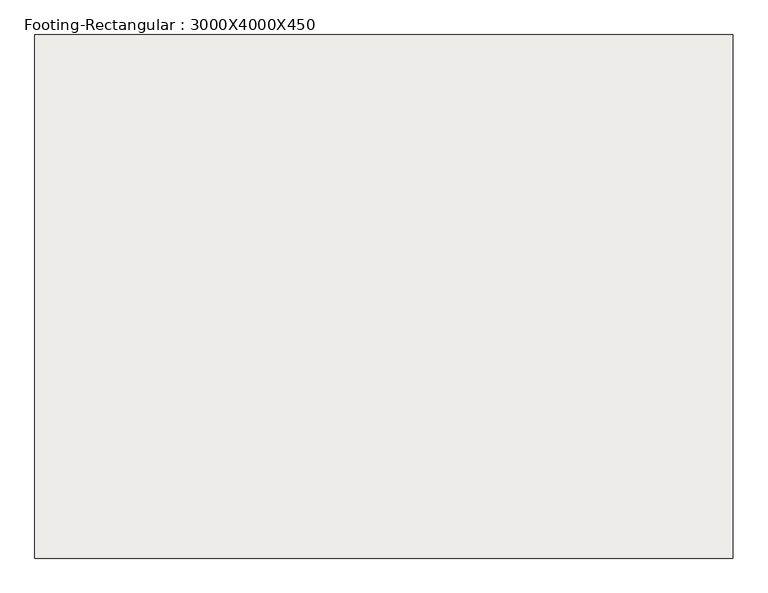
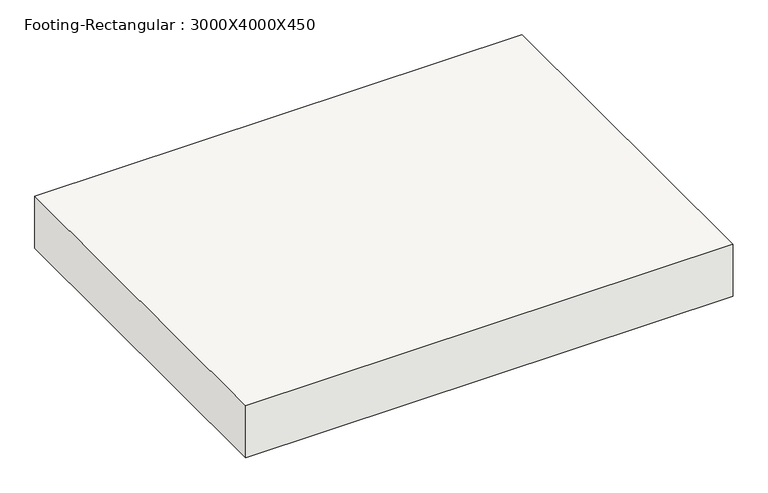
"""IFC4 building model written with IfcOpenShell, lengths in millimetres: slab geometry, Footing-Rectangular : 3000X4000X450."""

from ifc_helpers import new_model, si_unit, frame, origin, place, context, project, spatial, polyline, outline, extrude, source, transform, mapped, element, save


def footing_rectangular_3000x4000x450_ea1acd88(model_context):
    return source(origin(), model_context, "Body", "SweptSolid", [
        extrude(outline(polyline([(2000.0, 1500.0), (2000.0, -1500.0), (-2000.0, -1500.0), (-2000.0, 1500.0), (2000.0, 1500.0)])), frame((0.0, 0.0, -450.0), z_axis=(0.0, 0.0, 1.0), x_axis=(1.0, 0.0, 0.0)), (0.0, 0.0, 1.0), 450.0),
    ])


if __name__ == "__main__":
    model = new_model("IFC4")
    model_context = context("Model", 3, world=origin())
    ifc_project = project(units=[si_unit("LENGTHUNIT", "METRE", prefix="MILLI")], contexts=[model_context])
    site = spatial("IfcSite", under=ifc_project)
    building = spatial("IfcBuilding", under=site)
    placement = place(None, origin())
    footing_rectangular_3000x4000x450_shape = footing_rectangular_3000x4000x450_ea1acd88(model_context)
    element("IfcSlab", 1, ObjectType="Footing-Rectangular : 3000X4000X450", at=placement, inside=building, context=model_context, shape_type="MappedRepresentation", body=[
        mapped(footing_rectangular_3000x4000x450_shape, transform((0.0, 0.0, 0.0), x_axis=(1.0, 0.0, 0.0), y_axis=(0.0, 1.0, 0.0), z_axis=(0.0, 0.0, 1.0))),
    ])
    save(model, "model.ifc")

# Revit data of these elements
# Type "Footing-Rectangular : 3000X4000X450"
#   Width = 13' - 1.48031"
#   Length = 9' - 10.11024"
#   Foundation Thickness = 1' - 5.71654"
#   Structural Material [instance default] = Concrete - Cast-in-Place Concrete
#   Assembly Code = ""
# Element 1 (IfcSlab, "Footing-Rectangular : 3000X4000X450")
#   Materials on its faces: "Concrete - Cast-in-Place Concrete"
# Materials
#   "Concrete - Cast-in-Place Concrete": class "Concrete", colour RGB 192 192 192, transparency 0, Cost = 0
